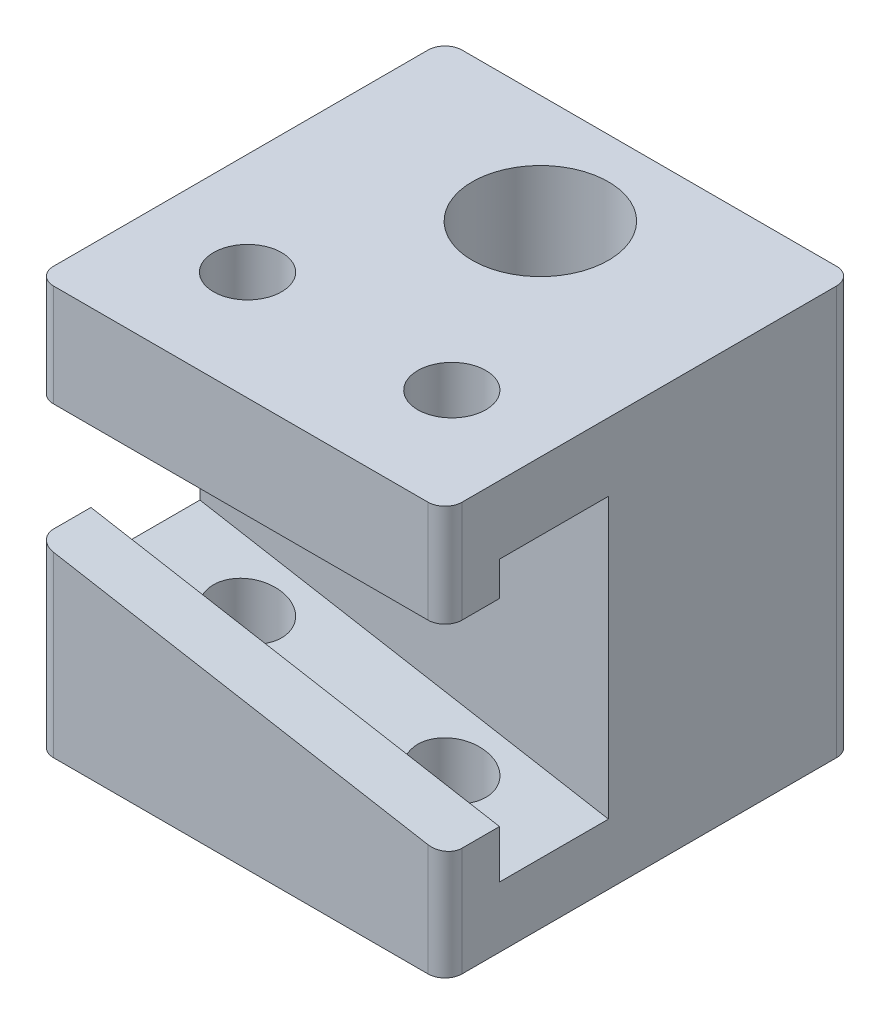
ISO-10303-21;
HEADER;
FILE_DESCRIPTION(('STEP AP214'),'2;1');
FILE_NAME('part.step','',(''),(''),'','','');
FILE_SCHEMA(('AUTOMOTIVE_DESIGN { 1 0 10303 214 1 1 1 1 }'));
ENDSEC;
DATA;
#1=APPLICATION_CONTEXT('core data for automotive mechanical design processes');
#2=APPLICATION_PROTOCOL_DEFINITION('international standard','automotive_design',2000,#1);
#3=PRODUCT_CONTEXT('',#1,'mechanical');
#4=PRODUCT('Part','Part','',(#3));
#5=PRODUCT_RELATED_PRODUCT_CATEGORY('part','',(#4));
#6=PRODUCT_DEFINITION_FORMATION('','',#4);
#7=PRODUCT_DEFINITION_CONTEXT('part definition',#1,'design');
#8=PRODUCT_DEFINITION('design','',#6,#7);
#9=PRODUCT_DEFINITION_SHAPE('','',#8);
#10=(LENGTH_UNIT() NAMED_UNIT(*) SI_UNIT(.MILLI.,.METRE.));
#11=(NAMED_UNIT(*) PLANE_ANGLE_UNIT() SI_UNIT($,.RADIAN.));
#12=(NAMED_UNIT(*) SI_UNIT($,.STERADIAN.) SOLID_ANGLE_UNIT());
#13=UNCERTAINTY_MEASURE_WITH_UNIT(LENGTH_MEASURE(1.E-05),#10,'distance_accuracy_value','');
#14=(GEOMETRIC_REPRESENTATION_CONTEXT(3) GLOBAL_UNCERTAINTY_ASSIGNED_CONTEXT((#13)) GLOBAL_UNIT_ASSIGNED_CONTEXT((#10,
#11,#12)) REPRESENTATION_CONTEXT('',''));
#15=CARTESIAN_POINT('',(0.,0.,0.));
#16=DIRECTION('',(0.,0.,1.));
#17=DIRECTION('',(1.,0.,0.));
#18=AXIS2_PLACEMENT_3D('',#15,#16,#17);
#19=CARTESIAN_POINT('',(1.5,1.5,1.5));
#20=DIRECTION('',(-1.,0.,0.));
#21=DIRECTION('',(0.,-1.,0.));
#22=AXIS2_PLACEMENT_3D('',#19,#20,#21);
#23=PLANE('',#22);
#24=DIRECTION('',(0.,0.,-1.));
#25=VECTOR('',#24,1.);
#26=CARTESIAN_POINT('',(1.5,-1.5,1.5));
#27=LINE('',#26,#25);
#28=CARTESIAN_POINT('',(1.5,-1.5,1.375));
#29=VERTEX_POINT('',#28);
#30=CARTESIAN_POINT('',(1.5,-1.5,-1.375));
#31=VERTEX_POINT('',#30);
#32=EDGE_CURVE('E243',#29,#31,#27,.T.);
#33=ORIENTED_EDGE('',*,*,#32,.T.);
#34=DIRECTION('',(0.,1.,0.));
#35=VECTOR('',#34,1.);
#36=CARTESIAN_POINT('',(1.5,1.5,-1.375));
#37=LINE('',#36,#35);
#38=CARTESIAN_POINT('',(1.5,1.5,-1.375));
#39=VERTEX_POINT('',#38);
#40=EDGE_CURVE('E286',#31,#39,#37,.T.);
#41=ORIENTED_EDGE('',*,*,#40,.T.);
#42=DIRECTION('',(0.,0.,-1.));
#43=VECTOR('',#42,1.);
#44=CARTESIAN_POINT('',(1.5,1.5,1.5));
#45=LINE('',#44,#43);
#46=CARTESIAN_POINT('',(1.5,1.5,1.375));
#47=VERTEX_POINT('',#46);
#48=EDGE_CURVE('E251',#47,#39,#45,.T.);
#49=ORIENTED_EDGE('',*,*,#48,.F.);
#50=DIRECTION('',(0.,1.,0.));
#51=VECTOR('',#50,1.);
#52=CARTESIAN_POINT('',(1.5,0.75,1.375));
#53=LINE('',#52,#51);
#54=CARTESIAN_POINT('',(1.5,0.75,1.375));
#55=VERTEX_POINT('',#54);
#56=EDGE_CURVE('E290',#47,#55,#53,.F.);
#57=ORIENTED_EDGE('',*,*,#56,.T.);
#58=DIRECTION('',(0.,0.,1.));
#59=VECTOR('',#58,1.);
#60=CARTESIAN_POINT('',(1.5,0.75,0.3));
#61=LINE('',#60,#59);
#62=CARTESIAN_POINT('',(1.5,0.75,1.1));
#63=VERTEX_POINT('',#62);
#64=EDGE_CURVE('E195',#63,#55,#61,.T.);
#65=ORIENTED_EDGE('',*,*,#64,.F.);
#66=DIRECTION('',(0.,1.,0.));
#67=VECTOR('',#66,1.);
#68=CARTESIAN_POINT('',(1.5,-0.7,1.1));
#69=LINE('',#68,#67);
#70=CARTESIAN_POINT('',(1.5,1.,1.1));
#71=VERTEX_POINT('',#70);
#72=EDGE_CURVE('E166',#63,#71,#69,.T.);
#73=ORIENTED_EDGE('',*,*,#72,.T.);
#74=DIRECTION('',(0.,0.,-1.));
#75=VECTOR('',#74,1.);
#76=CARTESIAN_POINT('',(1.5,1.,1.1));
#77=LINE('',#76,#75);
#78=CARTESIAN_POINT('',(1.5,1.,0.3));
#79=VERTEX_POINT('',#78);
#80=EDGE_CURVE('E182',#71,#79,#77,.T.);
#81=ORIENTED_EDGE('',*,*,#80,.T.);
#82=DIRECTION('',(0.,1.,0.));
#83=VECTOR('',#82,1.);
#84=CARTESIAN_POINT('',(1.5,0.75,0.3));
#85=LINE('',#84,#83);
#86=CARTESIAN_POINT('',(1.5,-1.053,0.3));
#87=VERTEX_POINT('',#86);
#88=EDGE_CURVE('E216',#87,#79,#85,.T.);
#89=ORIENTED_EDGE('',*,*,#88,.F.);
#90=DIRECTION('',(0.,0.,-1.));
#91=VECTOR('',#90,1.);
#92=CARTESIAN_POINT('',(1.5,-1.053,1.1));
#93=LINE('',#92,#91);
#94=CARTESIAN_POINT('',(1.5,-1.053,1.1));
#95=VERTEX_POINT('',#94);
#96=EDGE_CURVE('E206',#95,#87,#93,.T.);
#97=ORIENTED_EDGE('',*,*,#96,.F.);
#98=CARTESIAN_POINT('',(1.5,-0.7,1.1));
#99=VERTEX_POINT('',#98);
#100=EDGE_CURVE('E180',#95,#99,#69,.T.);
#101=ORIENTED_EDGE('',*,*,#100,.T.);
#102=DIRECTION('',(0.,0.,1.));
#103=VECTOR('',#102,1.);
#104=CARTESIAN_POINT('',(1.5,-0.7,0.3));
#105=LINE('',#104,#103);
#106=CARTESIAN_POINT('',(1.5,-0.7,1.375));
#107=VERTEX_POINT('',#106);
#108=EDGE_CURVE('E221',#99,#107,#105,.T.);
#109=ORIENTED_EDGE('',*,*,#108,.T.);
#110=DIRECTION('',(0.,1.,0.));
#111=VECTOR('',#110,1.);
#112=CARTESIAN_POINT('',(1.5,-1.5,1.375));
#113=LINE('',#112,#111);
#114=EDGE_CURVE('E284',#107,#29,#113,.F.);
#115=ORIENTED_EDGE('',*,*,#114,.T.);
#116=EDGE_LOOP('',(#33,#41,#49,#57,#65,#73,#81,#89,#97,#101,#109,#115));
#117=FACE_BOUND('',#116,.T.);
#118=ADVANCED_FACE('F39',(#117),#23,.F.);
#119=CARTESIAN_POINT('',(-1.5,1.5,1.5));
#120=DIRECTION('',(1.,0.,0.));
#121=DIRECTION('',(0.,1.,0.));
#122=AXIS2_PLACEMENT_3D('',#119,#120,#121);
#123=PLANE('',#122);
#124=DIRECTION('',(0.,0.,-1.));
#125=VECTOR('',#124,1.);
#126=CARTESIAN_POINT('',(-1.5,1.5,1.5));
#127=LINE('',#126,#125);
#128=CARTESIAN_POINT('',(-1.5,1.5,1.375));
#129=VERTEX_POINT('',#128);
#130=CARTESIAN_POINT('',(-1.5,1.5,-1.375));
#131=VERTEX_POINT('',#130);
#132=EDGE_CURVE('E248',#129,#131,#127,.T.);
#133=ORIENTED_EDGE('',*,*,#132,.T.);
#134=DIRECTION('',(0.,-1.,0.));
#135=VECTOR('',#134,1.);
#136=CARTESIAN_POINT('',(-1.5,1.5,-1.375));
#137=LINE('',#136,#135);
#138=CARTESIAN_POINT('',(-1.5,-1.5,-1.375));
#139=VERTEX_POINT('',#138);
#140=EDGE_CURVE('E265',#131,#139,#137,.T.);
#141=ORIENTED_EDGE('',*,*,#140,.T.);
#142=DIRECTION('',(0.,0.,-1.));
#143=VECTOR('',#142,1.);
#144=CARTESIAN_POINT('',(-1.5,-1.5,1.5));
#145=LINE('',#144,#143);
#146=CARTESIAN_POINT('',(-1.5,-1.5,1.375));
#147=VERTEX_POINT('',#146);
#148=EDGE_CURVE('E250',#147,#139,#145,.T.);
#149=ORIENTED_EDGE('',*,*,#148,.F.);
#150=DIRECTION('',(0.,-1.,0.));
#151=VECTOR('',#150,1.);
#152=CARTESIAN_POINT('',(-1.5,-0.171019057874627,1.375));
#153=LINE('',#152,#151);
#154=CARTESIAN_POINT('',(-1.5,-0.171019057874627,1.375));
#155=VERTEX_POINT('',#154);
#156=EDGE_CURVE('E256',#147,#155,#153,.F.);
#157=ORIENTED_EDGE('',*,*,#156,.T.);
#158=DIRECTION('',(0.,0.,1.));
#159=VECTOR('',#158,1.);
#160=CARTESIAN_POINT('',(-1.5,-0.171019057874627,0.3));
#161=LINE('',#160,#159);
#162=CARTESIAN_POINT('',(-1.5,-0.171019057874627,1.1));
#163=VERTEX_POINT('',#162);
#164=EDGE_CURVE('E226',#163,#155,#161,.T.);
#165=ORIENTED_EDGE('',*,*,#164,.F.);
#166=DIRECTION('',(0.,-1.,0.));
#167=VECTOR('',#166,1.);
#168=CARTESIAN_POINT('',(-1.5,-0.524019057874592,1.1));
#169=LINE('',#168,#167);
#170=CARTESIAN_POINT('',(-1.5,-0.524019057874592,1.1));
#171=VERTEX_POINT('',#170);
#172=EDGE_CURVE('E177',#163,#171,#169,.T.);
#173=ORIENTED_EDGE('',*,*,#172,.T.);
#174=DIRECTION('',(0.,0.,-1.));
#175=VECTOR('',#174,1.);
#176=CARTESIAN_POINT('',(-1.5,-0.524019057874592,1.1));
#177=LINE('',#176,#175);
#178=CARTESIAN_POINT('',(-1.5,-0.524019057874592,0.3));
#179=VERTEX_POINT('',#178);
#180=EDGE_CURVE('E209',#171,#179,#177,.T.);
#181=ORIENTED_EDGE('',*,*,#180,.T.);
#182=DIRECTION('',(0.,-1.,0.));
#183=VECTOR('',#182,1.);
#184=CARTESIAN_POINT('',(-1.5,0.75,0.3));
#185=LINE('',#184,#183);
#186=CARTESIAN_POINT('',(-1.5,1.,0.3));
#187=VERTEX_POINT('',#186);
#188=EDGE_CURVE('E217',#187,#179,#185,.T.);
#189=ORIENTED_EDGE('',*,*,#188,.F.);
#190=DIRECTION('',(0.,0.,-1.));
#191=VECTOR('',#190,1.);
#192=CARTESIAN_POINT('',(-1.5,1.,1.1));
#193=LINE('',#192,#191);
#194=CARTESIAN_POINT('',(-1.5,1.,1.1));
#195=VERTEX_POINT('',#194);
#196=EDGE_CURVE('E190',#195,#187,#193,.T.);
#197=ORIENTED_EDGE('',*,*,#196,.F.);
#198=CARTESIAN_POINT('',(-1.5,0.75,1.1));
#199=VERTEX_POINT('',#198);
#200=EDGE_CURVE('E175',#195,#199,#169,.T.);
#201=ORIENTED_EDGE('',*,*,#200,.T.);
#202=DIRECTION('',(0.,0.,1.));
#203=VECTOR('',#202,1.);
#204=CARTESIAN_POINT('',(-1.5,0.75,0.3));
#205=LINE('',#204,#203);
#206=CARTESIAN_POINT('',(-1.5,0.75,1.375));
#207=VERTEX_POINT('',#206);
#208=EDGE_CURVE('E229',#199,#207,#205,.T.);
#209=ORIENTED_EDGE('',*,*,#208,.T.);
#210=DIRECTION('',(0.,-1.,0.));
#211=VECTOR('',#210,1.);
#212=CARTESIAN_POINT('',(-1.5,1.5,1.375));
#213=LINE('',#212,#211);
#214=EDGE_CURVE('E257',#207,#129,#213,.F.);
#215=ORIENTED_EDGE('',*,*,#214,.T.);
#216=EDGE_LOOP('',(#133,#141,#149,#157,#165,#173,#181,#189,#197,#201,#209,#215));
#217=FACE_BOUND('',#216,.T.);
#218=ADVANCED_FACE('F357',(#217),#123,.F.);
#219=CARTESIAN_POINT('',(1.5,-0.7,0.3));
#220=DIRECTION('',(-0.173648177666923,-0.984807753012209,0.));
#221=DIRECTION('',(0.984807753012209,-0.173648177666923,0.));
#222=AXIS2_PLACEMENT_3D('',#219,#220,#221);
#223=PLANE('',#222);
#224=ORIENTED_EDGE('',*,*,#164,.T.);
#225=CARTESIAN_POINT('',(-1.375,-0.193059930463184,1.375));
#226=DIRECTION('',(-0.173648177666923,-0.984807753012209,0.));
#227=DIRECTION('',(-0.984807753012209,0.173648177666923,0.));
#228=AXIS2_PLACEMENT_3D('',#225,#226,#227);
#229=ELLIPSE('',#228,0.126928326485718,0.125);
#230=CARTESIAN_POINT('',(-1.375,-0.193059930463184,1.5));
#231=VERTEX_POINT('',#230);
#232=EDGE_CURVE('E11',#155,#231,#229,.F.);
#233=ORIENTED_EDGE('',*,*,#232,.T.);
#234=DIRECTION('',(0.984807753012209,-0.173648177666923,0.));
#235=VECTOR('',#234,1.);
#236=CARTESIAN_POINT('',(1.5,-0.7,1.5));
#237=LINE('',#236,#235);
#238=CARTESIAN_POINT('',(1.375,-0.677959127411443,1.5));
#239=VERTEX_POINT('',#238);
#240=EDGE_CURVE('E218',#231,#239,#237,.T.);
#241=ORIENTED_EDGE('',*,*,#240,.T.);
#242=CARTESIAN_POINT('',(1.375,-0.677959127411443,1.375));
#243=DIRECTION('',(-0.173648177666923,-0.984807753012209,0.));
#244=DIRECTION('',(0.984807753012209,-0.173648177666923,0.));
#245=AXIS2_PLACEMENT_3D('',#242,#243,#244);
#246=ELLIPSE('',#245,0.126928326485718,0.125);
#247=EDGE_CURVE('E48',#239,#107,#246,.F.);
#248=ORIENTED_EDGE('',*,*,#247,.T.);
#249=ORIENTED_EDGE('',*,*,#108,.F.);
#250=DIRECTION('',(0.984807753012209,-0.173648177666923,0.));
#251=VECTOR('',#250,1.);
#252=CARTESIAN_POINT('',(1.5,-0.7,1.1));
#253=LINE('',#252,#251);
#254=EDGE_CURVE('E188',#163,#99,#253,.T.);
#255=ORIENTED_EDGE('',*,*,#254,.F.);
#256=EDGE_LOOP('',(#224,#233,#241,#248,#249,#255));
#257=FACE_BOUND('',#256,.T.);
#258=ADVANCED_FACE('F362',(#257),#223,.F.);
#259=CARTESIAN_POINT('',(-1.5,0.75,0.3));
#260=DIRECTION('',(0.,1.,0.));
#261=DIRECTION('',(-1.,0.,0.));
#262=AXIS2_PLACEMENT_3D('',#259,#260,#261);
#263=PLANE('',#262);
#264=DIRECTION('',(-1.,0.,0.));
#265=VECTOR('',#264,1.);
#266=CARTESIAN_POINT('',(-1.5,0.75,1.5));
#267=LINE('',#266,#265);
#268=CARTESIAN_POINT('',(1.375,0.75,1.5));
#269=VERTEX_POINT('',#268);
#270=CARTESIAN_POINT('',(-1.375,0.75,1.5));
#271=VERTEX_POINT('',#270);
#272=EDGE_CURVE('E214',#269,#271,#267,.T.);
#273=ORIENTED_EDGE('',*,*,#272,.T.);
#274=CARTESIAN_POINT('',(-1.375,0.75,1.375));
#275=DIRECTION('',(0.,1.,0.));
#276=DIRECTION('',(-1.,0.,0.));
#277=AXIS2_PLACEMENT_3D('',#274,#275,#276);
#278=CIRCLE('',#277,0.125);
#279=EDGE_CURVE('E299',#271,#207,#278,.F.);
#280=ORIENTED_EDGE('',*,*,#279,.T.);
#281=ORIENTED_EDGE('',*,*,#208,.F.);
#282=DIRECTION('',(-1.,0.,0.));
#283=VECTOR('',#282,1.);
#284=CARTESIAN_POINT('',(-1.5,0.75,1.1));
#285=LINE('',#284,#283);
#286=EDGE_CURVE('E258',#63,#199,#285,.T.);
#287=ORIENTED_EDGE('',*,*,#286,.F.);
#288=ORIENTED_EDGE('',*,*,#64,.T.);
#289=CARTESIAN_POINT('',(1.375,0.75,1.375));
#290=DIRECTION('',(0.,1.,0.));
#291=DIRECTION('',(-1.,0.,0.));
#292=AXIS2_PLACEMENT_3D('',#289,#290,#291);
#293=CIRCLE('',#292,0.125);
#294=EDGE_CURVE('E296',#55,#269,#293,.F.);
#295=ORIENTED_EDGE('',*,*,#294,.T.);
#296=EDGE_LOOP('',(#273,#280,#281,#287,#288,#295));
#297=FACE_BOUND('',#296,.T.);
#298=ADVANCED_FACE('F391',(#297),#263,.F.);
#299=CARTESIAN_POINT('',(0.,0.,1.5));
#300=DIRECTION('',(0.,0.,1.));
#301=DIRECTION('',(1.,0.,0.));
#302=AXIS2_PLACEMENT_3D('',#299,#300,#301);
#303=PLANE('',#302);
#304=DIRECTION('',(-1.,0.,0.));
#305=VECTOR('',#304,1.);
#306=CARTESIAN_POINT('',(-1.5,1.5,1.5));
#307=LINE('',#306,#305);
#308=CARTESIAN_POINT('',(1.375,1.5,1.5));
#309=VERTEX_POINT('',#308);
#310=CARTESIAN_POINT('',(-1.375,1.5,1.5));
#311=VERTEX_POINT('',#310);
#312=EDGE_CURVE('E231',#309,#311,#307,.T.);
#313=ORIENTED_EDGE('',*,*,#312,.T.);
#314=DIRECTION('',(0.,-1.,0.));
#315=VECTOR('',#314,1.);
#316=CARTESIAN_POINT('',(-1.375,0.75,1.5));
#317=LINE('',#316,#315);
#318=EDGE_CURVE('E293',#311,#271,#317,.T.);
#319=ORIENTED_EDGE('',*,*,#318,.T.);
#320=ORIENTED_EDGE('',*,*,#272,.F.);
#321=DIRECTION('',(0.,1.,0.));
#322=VECTOR('',#321,1.);
#323=CARTESIAN_POINT('',(1.375,1.5,1.5));
#324=LINE('',#323,#322);
#325=EDGE_CURVE('E295',#269,#309,#324,.T.);
#326=ORIENTED_EDGE('',*,*,#325,.T.);
#327=EDGE_LOOP('',(#313,#319,#320,#326));
#328=FACE_BOUND('',#327,.T.);
#329=ADVANCED_FACE('F394',(#328),#303,.T.);
#330=CARTESIAN_POINT('',(-1.5,1.5,1.5));
#331=DIRECTION('',(0.,-1.,0.));
#332=DIRECTION('',(0.,0.,-1.));
#333=AXIS2_PLACEMENT_3D('',#330,#331,#332);
#334=PLANE('',#333);
#335=CARTESIAN_POINT('',(0.,1.5,-0.7));
#336=DIRECTION('',(0.,1.,0.));
#337=DIRECTION('',(0.,0.,1.));
#338=AXIS2_PLACEMENT_3D('',#335,#336,#337);
#339=CIRCLE('',#338,0.5);
#340=CARTESIAN_POINT('',(0.,1.5,-0.2));
#341=VERTEX_POINT('',#340);
#342=EDGE_CURVE('E312',#341,#341,#339,.T.);
#343=ORIENTED_EDGE('',*,*,#342,.F.);
#344=EDGE_LOOP('',(#343));
#345=FACE_BOUND('',#344,.T.);
#346=CARTESIAN_POINT('',(0.75,1.5,0.7));
#347=DIRECTION('',(0.,1.,0.));
#348=DIRECTION('',(0.,0.,1.));
#349=AXIS2_PLACEMENT_3D('',#346,#347,#348);
#350=CIRCLE('',#349,0.25);
#351=CARTESIAN_POINT('',(0.75,1.5,0.95));
#352=VERTEX_POINT('',#351);
#353=EDGE_CURVE('E319',#352,#352,#350,.T.);
#354=ORIENTED_EDGE('',*,*,#353,.F.);
#355=EDGE_LOOP('',(#354));
#356=FACE_BOUND('',#355,.T.);
#357=CARTESIAN_POINT('',(-0.75,1.5,0.7));
#358=DIRECTION('',(0.,1.,0.));
#359=DIRECTION('',(0.,0.,1.));
#360=AXIS2_PLACEMENT_3D('',#357,#358,#359);
#361=CIRCLE('',#360,0.25);
#362=CARTESIAN_POINT('',(-0.75,1.5,0.95));
#363=VERTEX_POINT('',#362);
#364=EDGE_CURVE('E327',#363,#363,#361,.T.);
#365=ORIENTED_EDGE('',*,*,#364,.F.);
#366=EDGE_LOOP('',(#365));
#367=FACE_BOUND('',#366,.T.);
#368=DIRECTION('',(-1.,0.,0.));
#369=VECTOR('',#368,1.);
#370=CARTESIAN_POINT('',(-1.5,1.5,-1.5));
#371=LINE('',#370,#369);
#372=CARTESIAN_POINT('',(1.375,1.5,-1.5));
#373=VERTEX_POINT('',#372);
#374=CARTESIAN_POINT('',(-1.375,1.5,-1.5));
#375=VERTEX_POINT('',#374);
#376=EDGE_CURVE('E230',#373,#375,#371,.T.);
#377=ORIENTED_EDGE('',*,*,#376,.T.);
#378=CARTESIAN_POINT('',(-1.375,1.5,-1.375));
#379=DIRECTION('',(0.,-1.,0.));
#380=DIRECTION('',(0.,0.,-1.));
#381=AXIS2_PLACEMENT_3D('',#378,#379,#380);
#382=CIRCLE('',#381,0.125);
#383=EDGE_CURVE('E281',#375,#131,#382,.F.);
#384=ORIENTED_EDGE('',*,*,#383,.T.);
#385=ORIENTED_EDGE('',*,*,#132,.F.);
#386=CARTESIAN_POINT('',(-1.375,1.5,1.375));
#387=DIRECTION('',(0.,-1.,0.));
#388=DIRECTION('',(0.,0.,-1.));
#389=AXIS2_PLACEMENT_3D('',#386,#387,#388);
#390=CIRCLE('',#389,0.125);
#391=EDGE_CURVE('E276',#129,#311,#390,.F.);
#392=ORIENTED_EDGE('',*,*,#391,.T.);
#393=ORIENTED_EDGE('',*,*,#312,.F.);
#394=CARTESIAN_POINT('',(1.375,1.5,1.375));
#395=DIRECTION('',(0.,-1.,0.));
#396=DIRECTION('',(0.,0.,-1.));
#397=AXIS2_PLACEMENT_3D('',#394,#395,#396);
#398=CIRCLE('',#397,0.125);
#399=EDGE_CURVE('E280',#309,#47,#398,.F.);
#400=ORIENTED_EDGE('',*,*,#399,.T.);
#401=ORIENTED_EDGE('',*,*,#48,.T.);
#402=CARTESIAN_POINT('',(1.375,1.5,-1.375));
#403=DIRECTION('',(0.,-1.,0.));
#404=DIRECTION('',(0.,0.,-1.));
#405=AXIS2_PLACEMENT_3D('',#402,#403,#404);
#406=CIRCLE('',#405,0.125);
#407=EDGE_CURVE('E283',#39,#373,#406,.F.);
#408=ORIENTED_EDGE('',*,*,#407,.T.);
#409=EDGE_LOOP('',(#377,#384,#385,#392,#393,#400,#401,#408));
#410=FACE_BOUND('',#409,.T.);
#411=ADVANCED_FACE('F370',(#345,#356,#367,#410),#334,.F.);
#412=CARTESIAN_POINT('',(-1.5,-1.5,1.5));
#413=DIRECTION('',(0.,1.,0.));
#414=DIRECTION('',(0.,0.,1.));
#415=AXIS2_PLACEMENT_3D('',#412,#413,#414);
#416=PLANE('',#415);
#417=CARTESIAN_POINT('',(0.,-1.5,-0.7));
#418=DIRECTION('',(0.,1.,0.));
#419=DIRECTION('',(0.,0.,1.));
#420=AXIS2_PLACEMENT_3D('',#417,#418,#419);
#421=CIRCLE('',#420,0.5);
#422=CARTESIAN_POINT('',(0.,-1.5,-0.2));
#423=VERTEX_POINT('',#422);
#424=EDGE_CURVE('E309',#423,#423,#421,.T.);
#425=ORIENTED_EDGE('',*,*,#424,.T.);
#426=EDGE_LOOP('',(#425));
#427=FACE_BOUND('',#426,.T.);
#428=CARTESIAN_POINT('',(0.75,-1.5,0.7));
#429=DIRECTION('',(0.,1.,0.));
#430=DIRECTION('',(0.,0.,1.));
#431=AXIS2_PLACEMENT_3D('',#428,#429,#430);
#432=CIRCLE('',#431,0.25);
#433=CARTESIAN_POINT('',(0.75,-1.5,0.95));
#434=VERTEX_POINT('',#433);
#435=EDGE_CURVE('E324',#434,#434,#432,.T.);
#436=ORIENTED_EDGE('',*,*,#435,.T.);
#437=EDGE_LOOP('',(#436));
#438=FACE_BOUND('',#437,.T.);
#439=CARTESIAN_POINT('',(-0.75,-1.5,0.7));
#440=DIRECTION('',(0.,1.,0.));
#441=DIRECTION('',(0.,0.,1.));
#442=AXIS2_PLACEMENT_3D('',#439,#440,#441);
#443=CIRCLE('',#442,0.25);
#444=CARTESIAN_POINT('',(-0.75,-1.5,0.95));
#445=VERTEX_POINT('',#444);
#446=EDGE_CURVE('E332',#445,#445,#443,.T.);
#447=ORIENTED_EDGE('',*,*,#446,.T.);
#448=EDGE_LOOP('',(#447));
#449=FACE_BOUND('',#448,.T.);
#450=ORIENTED_EDGE('',*,*,#148,.T.);
#451=CARTESIAN_POINT('',(-1.375,-1.5,-1.375));
#452=DIRECTION('',(0.,1.,0.));
#453=DIRECTION('',(0.,0.,1.));
#454=AXIS2_PLACEMENT_3D('',#451,#452,#453);
#455=CIRCLE('',#454,0.125);
#456=CARTESIAN_POINT('',(-1.375,-1.5,-1.5));
#457=VERTEX_POINT('',#456);
#458=EDGE_CURVE('E271',#139,#457,#455,.F.);
#459=ORIENTED_EDGE('',*,*,#458,.T.);
#460=DIRECTION('',(1.,0.,0.));
#461=VECTOR('',#460,1.);
#462=CARTESIAN_POINT('',(-1.5,-1.5,-1.5));
#463=LINE('',#462,#461);
#464=CARTESIAN_POINT('',(1.375,-1.5,-1.5));
#465=VERTEX_POINT('',#464);
#466=EDGE_CURVE('E236',#457,#465,#463,.T.);
#467=ORIENTED_EDGE('',*,*,#466,.T.);
#468=CARTESIAN_POINT('',(1.375,-1.5,-1.375));
#469=DIRECTION('',(0.,1.,0.));
#470=DIRECTION('',(0.,0.,1.));
#471=AXIS2_PLACEMENT_3D('',#468,#469,#470);
#472=CIRCLE('',#471,0.125);
#473=EDGE_CURVE('E267',#465,#31,#472,.F.);
#474=ORIENTED_EDGE('',*,*,#473,.T.);
#475=ORIENTED_EDGE('',*,*,#32,.F.);
#476=CARTESIAN_POINT('',(1.375,-1.5,1.375));
#477=DIRECTION('',(0.,1.,0.));
#478=DIRECTION('',(0.,0.,1.));
#479=AXIS2_PLACEMENT_3D('',#476,#477,#478);
#480=CIRCLE('',#479,0.125);
#481=CARTESIAN_POINT('',(1.375,-1.5,1.5));
#482=VERTEX_POINT('',#481);
#483=EDGE_CURVE('E264',#29,#482,#480,.F.);
#484=ORIENTED_EDGE('',*,*,#483,.T.);
#485=DIRECTION('',(1.,0.,0.));
#486=VECTOR('',#485,1.);
#487=CARTESIAN_POINT('',(-1.5,-1.5,1.5));
#488=LINE('',#487,#486);
#489=CARTESIAN_POINT('',(-1.375,-1.5,1.5));
#490=VERTEX_POINT('',#489);
#491=EDGE_CURVE('E240',#490,#482,#488,.T.);
#492=ORIENTED_EDGE('',*,*,#491,.F.);
#493=CARTESIAN_POINT('',(-1.375,-1.5,1.375));
#494=DIRECTION('',(0.,1.,0.));
#495=DIRECTION('',(0.,0.,1.));
#496=AXIS2_PLACEMENT_3D('',#493,#494,#495);
#497=CIRCLE('',#496,0.125);
#498=EDGE_CURVE('E270',#490,#147,#497,.F.);
#499=ORIENTED_EDGE('',*,*,#498,.T.);
#500=EDGE_LOOP('',(#450,#459,#467,#474,#475,#484,#492,#499));
#501=FACE_BOUND('',#500,.T.);
#502=ADVANCED_FACE('F333',(#427,#438,#449,#501),#416,.F.);
#503=ORIENTED_EDGE('',*,*,#240,.F.);
#504=DIRECTION('',(0.,-1.,0.));
#505=VECTOR('',#504,1.);
#506=CARTESIAN_POINT('',(-1.375,-1.5,1.5));
#507=LINE('',#506,#505);
#508=EDGE_CURVE('E301',#231,#490,#507,.T.);
#509=ORIENTED_EDGE('',*,*,#508,.T.);
#510=ORIENTED_EDGE('',*,*,#491,.T.);
#511=DIRECTION('',(0.,1.,0.));
#512=VECTOR('',#511,1.);
#513=CARTESIAN_POINT('',(1.375,-0.7,1.5));
#514=LINE('',#513,#512);
#515=EDGE_CURVE('E305',#482,#239,#514,.T.);
#516=ORIENTED_EDGE('',*,*,#515,.T.);
#517=EDGE_LOOP('',(#503,#509,#510,#516));
#518=FACE_BOUND('',#517,.T.);
#519=ADVANCED_FACE('F420',(#518),#303,.T.);
#520=CARTESIAN_POINT('',(0.,0.,-1.5));
#521=DIRECTION('',(0.,0.,1.));
#522=DIRECTION('',(1.,0.,0.));
#523=AXIS2_PLACEMENT_3D('',#520,#521,#522);
#524=PLANE('',#523);
#525=ORIENTED_EDGE('',*,*,#466,.F.);
#526=DIRECTION('',(0.,-1.,0.));
#527=VECTOR('',#526,1.);
#528=CARTESIAN_POINT('',(-1.375,0.,-1.5));
#529=LINE('',#528,#527);
#530=EDGE_CURVE('E274',#457,#375,#529,.F.);
#531=ORIENTED_EDGE('',*,*,#530,.T.);
#532=ORIENTED_EDGE('',*,*,#376,.F.);
#533=DIRECTION('',(0.,1.,0.));
#534=VECTOR('',#533,1.);
#535=CARTESIAN_POINT('',(1.375,0.,-1.5));
#536=LINE('',#535,#534);
#537=EDGE_CURVE('E272',#373,#465,#536,.F.);
#538=ORIENTED_EDGE('',*,*,#537,.T.);
#539=EDGE_LOOP('',(#525,#531,#532,#538));
#540=FACE_BOUND('',#539,.T.);
#541=ADVANCED_FACE('F431',(#540),#524,.F.);
#542=CARTESIAN_POINT('',(0.,0.,0.3));
#543=DIRECTION('',(0.,0.,1.));
#544=DIRECTION('',(1.,0.,0.));
#545=AXIS2_PLACEMENT_3D('',#542,#543,#544);
#546=PLANE('',#545);
#547=ORIENTED_EDGE('',*,*,#88,.T.);
#548=DIRECTION('',(-1.,0.,0.));
#549=VECTOR('',#548,1.);
#550=CARTESIAN_POINT('',(-1.5,1.,0.3));
#551=LINE('',#550,#549);
#552=EDGE_CURVE('E184',#79,#187,#551,.T.);
#553=ORIENTED_EDGE('',*,*,#552,.T.);
#554=ORIENTED_EDGE('',*,*,#188,.T.);
#555=DIRECTION('',(0.984807753012207,-0.173648177666934,0.));
#556=VECTOR('',#555,1.);
#557=CARTESIAN_POINT('',(-1.5,-0.524019057874592,0.3));
#558=LINE('',#557,#556);
#559=EDGE_CURVE('E194',#179,#87,#558,.T.);
#560=ORIENTED_EDGE('',*,*,#559,.T.);
#561=EDGE_LOOP('',(#547,#553,#554,#560));
#562=FACE_BOUND('',#561,.T.);
#563=ADVANCED_FACE('F403',(#562),#546,.T.);
#564=CARTESIAN_POINT('',(0.,0.,1.1));
#565=DIRECTION('',(0.,0.,-1.));
#566=DIRECTION('',(-1.,0.,0.));
#567=AXIS2_PLACEMENT_3D('',#564,#565,#566);
#568=PLANE('',#567);
#569=ORIENTED_EDGE('',*,*,#286,.T.);
#570=ORIENTED_EDGE('',*,*,#200,.F.);
#571=DIRECTION('',(-1.,0.,0.));
#572=VECTOR('',#571,1.);
#573=CARTESIAN_POINT('',(-1.5,1.,1.1));
#574=LINE('',#573,#572);
#575=EDGE_CURVE('E164',#71,#195,#574,.T.);
#576=ORIENTED_EDGE('',*,*,#575,.F.);
#577=ORIENTED_EDGE('',*,*,#72,.F.);
#578=EDGE_LOOP('',(#569,#570,#576,#577));
#579=FACE_BOUND('',#578,.T.);
#580=ADVANCED_FACE('F170',(#579),#568,.T.);
#581=CARTESIAN_POINT('',(-1.5,1.,1.1));
#582=DIRECTION('',(0.,-1.,0.));
#583=DIRECTION('',(0.,0.,-1.));
#584=AXIS2_PLACEMENT_3D('',#581,#582,#583);
#585=PLANE('',#584);
#586=CARTESIAN_POINT('',(0.75,1.,0.7));
#587=DIRECTION('',(0.,-1.,0.));
#588=DIRECTION('',(0.,0.,-1.));
#589=AXIS2_PLACEMENT_3D('',#586,#587,#588);
#590=CIRCLE('',#589,0.25);
#591=CARTESIAN_POINT('',(0.75,1.,0.45));
#592=VERTEX_POINT('',#591);
#593=EDGE_CURVE('E200',#592,#592,#590,.T.);
#594=ORIENTED_EDGE('',*,*,#593,.F.);
#595=EDGE_LOOP('',(#594));
#596=FACE_BOUND('',#595,.T.);
#597=CARTESIAN_POINT('',(-0.75,1.,0.7));
#598=DIRECTION('',(0.,-1.,0.));
#599=DIRECTION('',(0.,0.,-1.));
#600=AXIS2_PLACEMENT_3D('',#597,#598,#599);
#601=CIRCLE('',#600,0.25);
#602=CARTESIAN_POINT('',(-0.75,1.,0.45));
#603=VERTEX_POINT('',#602);
#604=EDGE_CURVE('E310',#603,#603,#601,.T.);
#605=ORIENTED_EDGE('',*,*,#604,.F.);
#606=EDGE_LOOP('',(#605));
#607=FACE_BOUND('',#606,.T.);
#608=ORIENTED_EDGE('',*,*,#552,.F.);
#609=ORIENTED_EDGE('',*,*,#80,.F.);
#610=ORIENTED_EDGE('',*,*,#575,.T.);
#611=ORIENTED_EDGE('',*,*,#196,.T.);
#612=EDGE_LOOP('',(#608,#609,#610,#611));
#613=FACE_BOUND('',#612,.T.);
#614=ADVANCED_FACE('F185',(#596,#607,#613),#585,.T.);
#615=ORIENTED_EDGE('',*,*,#254,.T.);
#616=ORIENTED_EDGE('',*,*,#100,.F.);
#617=DIRECTION('',(0.984807753012207,-0.173648177666934,0.));
#618=VECTOR('',#617,1.);
#619=CARTESIAN_POINT('',(-1.5,-0.524019057874592,1.1));
#620=LINE('',#619,#618);
#621=EDGE_CURVE('E201',#171,#95,#620,.T.);
#622=ORIENTED_EDGE('',*,*,#621,.F.);
#623=ORIENTED_EDGE('',*,*,#172,.F.);
#624=EDGE_LOOP('',(#615,#616,#622,#623));
#625=FACE_BOUND('',#624,.T.);
#626=ADVANCED_FACE('F412',(#625),#568,.T.);
#627=CARTESIAN_POINT('',(-1.5,-0.524019057874592,1.1));
#628=DIRECTION('',(0.173648177666934,0.984807753012207,0.));
#629=DIRECTION('',(-0.984807753012207,0.173648177666934,0.));
#630=AXIS2_PLACEMENT_3D('',#627,#628,#629);
#631=PLANE('',#630);
#632=CARTESIAN_POINT('',(0.75,-0.920754764468648,0.7));
#633=DIRECTION('',(0.173648177666934,0.984807753012207,0.));
#634=DIRECTION('',(-0.984807753012207,0.173648177666934,0.));
#635=AXIS2_PLACEMENT_3D('',#632,#633,#634);
#636=ELLIPSE('',#635,0.253856652971436,0.25);
#637=CARTESIAN_POINT('',(0.5,-0.876673019291531,0.7));
#638=VERTEX_POINT('',#637);
#639=EDGE_CURVE('E43',#638,#638,#636,.T.);
#640=ORIENTED_EDGE('',*,*,#639,.F.);
#641=EDGE_LOOP('',(#640));
#642=FACE_BOUND('',#641,.T.);
#643=CARTESIAN_POINT('',(-0.75,-0.656264293405944,0.7));
#644=DIRECTION('',(0.173648177666934,0.984807753012207,0.));
#645=DIRECTION('',(-0.984807753012207,0.173648177666934,0.));
#646=AXIS2_PLACEMENT_3D('',#643,#644,#645);
#647=ELLIPSE('',#646,0.253856652971436,0.25);
#648=CARTESIAN_POINT('',(-1.,-0.612182548228827,0.7));
#649=VERTEX_POINT('',#648);
#650=EDGE_CURVE('E307',#649,#649,#647,.T.);
#651=ORIENTED_EDGE('',*,*,#650,.F.);
#652=EDGE_LOOP('',(#651));
#653=FACE_BOUND('',#652,.T.);
#654=ORIENTED_EDGE('',*,*,#559,.F.);
#655=ORIENTED_EDGE('',*,*,#180,.F.);
#656=ORIENTED_EDGE('',*,*,#621,.T.);
#657=ORIENTED_EDGE('',*,*,#96,.T.);
#658=EDGE_LOOP('',(#654,#655,#656,#657));
#659=FACE_BOUND('',#658,.T.);
#660=ADVANCED_FACE('F375',(#642,#653,#659),#631,.T.);
#661=CARTESIAN_POINT('',(-1.375,1.5,-1.375));
#662=DIRECTION('',(0.,-1.,0.));
#663=DIRECTION('',(1.,0.,0.));
#664=AXIS2_PLACEMENT_3D('',#661,#662,#663);
#665=CYLINDRICAL_SURFACE('',#664,0.125);
#666=ORIENTED_EDGE('',*,*,#383,.F.);
#667=ORIENTED_EDGE('',*,*,#530,.F.);
#668=ORIENTED_EDGE('',*,*,#458,.F.);
#669=ORIENTED_EDGE('',*,*,#140,.F.);
#670=EDGE_LOOP('',(#666,#667,#668,#669));
#671=FACE_BOUND('',#670,.T.);
#672=ADVANCED_FACE('F366',(#671),#665,.T.);
#673=CARTESIAN_POINT('',(1.375,1.5,-1.375));
#674=DIRECTION('',(0.,1.,0.));
#675=DIRECTION('',(-1.,0.,0.));
#676=AXIS2_PLACEMENT_3D('',#673,#674,#675);
#677=CYLINDRICAL_SURFACE('',#676,0.125);
#678=ORIENTED_EDGE('',*,*,#473,.F.);
#679=ORIENTED_EDGE('',*,*,#537,.F.);
#680=ORIENTED_EDGE('',*,*,#407,.F.);
#681=ORIENTED_EDGE('',*,*,#40,.F.);
#682=EDGE_LOOP('',(#678,#679,#680,#681));
#683=FACE_BOUND('',#682,.T.);
#684=ADVANCED_FACE('F371',(#683),#677,.T.);
#685=CARTESIAN_POINT('',(-1.375,0.,1.375));
#686=DIRECTION('',(0.,1.,0.));
#687=DIRECTION('',(-1.,0.,0.));
#688=AXIS2_PLACEMENT_3D('',#685,#686,#687);
#689=CYLINDRICAL_SURFACE('',#688,0.125);
#690=ORIENTED_EDGE('',*,*,#391,.F.);
#691=ORIENTED_EDGE('',*,*,#214,.F.);
#692=ORIENTED_EDGE('',*,*,#279,.F.);
#693=ORIENTED_EDGE('',*,*,#318,.F.);
#694=EDGE_LOOP('',(#690,#691,#692,#693));
#695=FACE_BOUND('',#694,.T.);
#696=ADVANCED_FACE('F376',(#695),#689,.T.);
#697=CARTESIAN_POINT('',(-1.375,0.,1.375));
#698=DIRECTION('',(0.,1.,0.));
#699=DIRECTION('',(-1.,0.,0.));
#700=AXIS2_PLACEMENT_3D('',#697,#698,#699);
#701=CYLINDRICAL_SURFACE('',#700,0.125);
#702=ORIENTED_EDGE('',*,*,#232,.F.);
#703=ORIENTED_EDGE('',*,*,#156,.F.);
#704=ORIENTED_EDGE('',*,*,#498,.F.);
#705=ORIENTED_EDGE('',*,*,#508,.F.);
#706=EDGE_LOOP('',(#702,#703,#704,#705));
#707=FACE_BOUND('',#706,.T.);
#708=ADVANCED_FACE('F379',(#707),#701,.T.);
#709=CARTESIAN_POINT('',(1.375,0.,1.375));
#710=DIRECTION('',(0.,-1.,0.));
#711=DIRECTION('',(1.,0.,0.));
#712=AXIS2_PLACEMENT_3D('',#709,#710,#711);
#713=CYLINDRICAL_SURFACE('',#712,0.125);
#714=ORIENTED_EDGE('',*,*,#294,.F.);
#715=ORIENTED_EDGE('',*,*,#56,.F.);
#716=ORIENTED_EDGE('',*,*,#399,.F.);
#717=ORIENTED_EDGE('',*,*,#325,.F.);
#718=EDGE_LOOP('',(#714,#715,#716,#717));
#719=FACE_BOUND('',#718,.T.);
#720=ADVANCED_FACE('F353',(#719),#713,.T.);
#721=CARTESIAN_POINT('',(1.375,0.,1.375));
#722=DIRECTION('',(0.,-1.,0.));
#723=DIRECTION('',(1.,0.,0.));
#724=AXIS2_PLACEMENT_3D('',#721,#722,#723);
#725=CYLINDRICAL_SURFACE('',#724,0.125);
#726=ORIENTED_EDGE('',*,*,#483,.F.);
#727=ORIENTED_EDGE('',*,*,#114,.F.);
#728=ORIENTED_EDGE('',*,*,#247,.F.);
#729=ORIENTED_EDGE('',*,*,#515,.F.);
#730=EDGE_LOOP('',(#726,#727,#728,#729));
#731=FACE_BOUND('',#730,.T.);
#732=ADVANCED_FACE('F41',(#731),#725,.T.);
#733=CARTESIAN_POINT('',(-0.75,-1.5,0.7));
#734=DIRECTION('',(0.,1.,0.));
#735=DIRECTION('',(0.,0.,1.));
#736=AXIS2_PLACEMENT_3D('',#733,#734,#735);
#737=CYLINDRICAL_SURFACE('',#736,0.25);
#738=ORIENTED_EDGE('',*,*,#650,.T.);
#739=EDGE_LOOP('',(#738));
#740=FACE_BOUND('',#739,.T.);
#741=ORIENTED_EDGE('',*,*,#446,.F.);
#742=EDGE_LOOP('',(#741));
#743=FACE_BOUND('',#742,.T.);
#744=ADVANCED_FACE('F336',(#740,#743),#737,.F.);
#745=CARTESIAN_POINT('',(0.75,-1.5,0.7));
#746=DIRECTION('',(0.,1.,0.));
#747=DIRECTION('',(0.,0.,1.));
#748=AXIS2_PLACEMENT_3D('',#745,#746,#747);
#749=CYLINDRICAL_SURFACE('',#748,0.25);
#750=ORIENTED_EDGE('',*,*,#639,.T.);
#751=EDGE_LOOP('',(#750));
#752=FACE_BOUND('',#751,.T.);
#753=ORIENTED_EDGE('',*,*,#435,.F.);
#754=EDGE_LOOP('',(#753));
#755=FACE_BOUND('',#754,.T.);
#756=ADVANCED_FACE('F339',(#752,#755),#749,.F.);
#757=ORIENTED_EDGE('',*,*,#604,.T.);
#758=EDGE_LOOP('',(#757));
#759=FACE_BOUND('',#758,.T.);
#760=ORIENTED_EDGE('',*,*,#364,.T.);
#761=EDGE_LOOP('',(#760));
#762=FACE_BOUND('',#761,.T.);
#763=ADVANCED_FACE('F345',(#759,#762),#737,.F.);
#764=ORIENTED_EDGE('',*,*,#593,.T.);
#765=EDGE_LOOP('',(#764));
#766=FACE_BOUND('',#765,.T.);
#767=ORIENTED_EDGE('',*,*,#353,.T.);
#768=EDGE_LOOP('',(#767));
#769=FACE_BOUND('',#768,.T.);
#770=ADVANCED_FACE('F349',(#766,#769),#749,.F.);
#771=CARTESIAN_POINT('',(0.,-1.5,-0.7));
#772=DIRECTION('',(0.,1.,0.));
#773=DIRECTION('',(0.,0.,1.));
#774=AXIS2_PLACEMENT_3D('',#771,#772,#773);
#775=CYLINDRICAL_SURFACE('',#774,0.5);
#776=ORIENTED_EDGE('',*,*,#424,.F.);
#777=EDGE_LOOP('',(#776));
#778=FACE_BOUND('',#777,.T.);
#779=ORIENTED_EDGE('',*,*,#342,.T.);
#780=EDGE_LOOP('',(#779));
#781=FACE_BOUND('',#780,.T.);
#782=ADVANCED_FACE('F462',(#778,#781),#775,.F.);
#783=CLOSED_SHELL('',(#118,#218,#258,#298,#329,#411,#502,#519,#541,#563,#580,#614,#626,#660,
#672,#684,#696,#708,#720,#732,#744,#756,#763,#770,#782));
#784=MANIFOLD_SOLID_BREP('B2',#783);
#785=ADVANCED_BREP_SHAPE_REPRESENTATION('',(#18,#784),#14);
#786=SHAPE_DEFINITION_REPRESENTATION(#9,#785);
ENDSEC;
END-ISO-10303-21;
